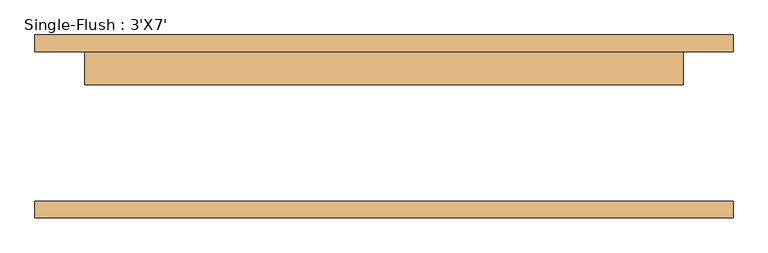
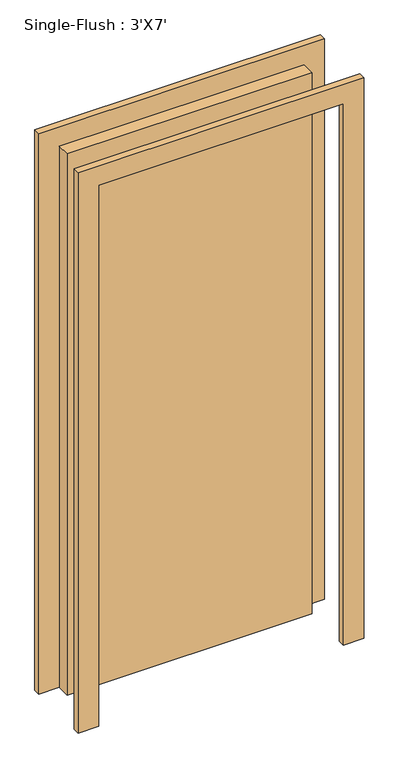
"""IFC4 building model written with IfcOpenShell, lengths in millimetres: door geometry, Single-Flush : 3'X7'."""

from ifc_helpers import new_model, si_unit, frame, origin, origin_with_axes, place, context, project, spatial, polyline, outline, extrude, source, transform, mapped, element, save


def single_flush_3_x7_0ca8825f(model_context):
    return source(origin(), model_context, "Body", "SweptSolid", [
        extrude(outline(polyline([(2209.8, -533.4), (0.0, -533.4), (0.0, -457.2), (2133.6, -457.2), (2133.6, 457.2), (0.0, 457.2), (0.0, 533.4), (2209.8, 533.4), (2209.8, -533.4)])), frame((0.0, 114.3, 0.0), z_axis=(0.0, 1.0, 0.0), x_axis=(0.0, 0.0, 1.0)), (0.0, 0.0, 1.0), 25.4),
        extrude(outline(polyline([(2209.8, 533.4), (2209.8, -533.4), (0.0, -533.4), (0.0, -457.2), (2133.6, -457.2), (2133.6, 457.2), (0.0, 457.2), (0.0, 533.4), (2209.8, 533.4)])), frame((0.0, -139.7, 0.0), z_axis=(0.0, 1.0, 0.0), x_axis=(0.0, 0.0, 1.0)), (0.0, 0.0, 1.0), 25.4),
        extrude(outline(polyline([(457.2, 63.5), (-457.2, 63.5), (-457.2, 114.3), (457.2, 114.3), (457.2, 63.5)])), origin_with_axes(), (0.0, 0.0, 1.0), 2133.6),
    ])


if __name__ == "__main__":
    model = new_model("IFC4")
    model_context = context("Model", 3, world=origin())
    ifc_project = project(units=[si_unit("LENGTHUNIT", "METRE", prefix="MILLI")], contexts=[model_context])
    site = spatial("IfcSite", under=ifc_project)
    building = spatial("IfcBuilding", under=site)
    placement = place(None, origin())
    single_flush_3_x7_shape = single_flush_3_x7_0ca8825f(model_context)
    element("IfcDoor", 1, ObjectType="Single-Flush : 3'X7'", at=placement, inside=building, context=model_context, shape_type="MappedRepresentation", body=[
        mapped(single_flush_3_x7_shape, transform((0.0, 0.0, 0.0), x_axis=(1.0, 0.0, 0.0), y_axis=(0.0, 1.0, 0.0), z_axis=(0.0, 0.0, 1.0))),
    ])
    save(model, "model.ifc")

# Revit data of these elements
# Type "Single-Flush : 3'X7'"
#   Type Mark = "8"
#   Construction Type Id = "MDOOR"
#   Assembly Code = "C1020"
#   Analytic Construction = "Metal"
#   Thickness = 0' - 2"
#   Heat Transfer Coefficient (U) = 0.651978 BTU/(h·ft²·°F)
#   Height = 7' - 0"
#   Trim Projection Ext = 0' - 1"
#   Trim Projection Int = 0' - 1"
#   Trim Width = 0' - 3"
#   Width = 3' - 0"
#   Define Thermal Properties by = 1
#   Door Material = Door - Panel
#   Frame Material = Door - Frame
#   Visual Light Transmittance = 0
#   Solar Heat Gain Coefficient = 0
#   Function = (empty or 0)
#   Wall Closure = (empty or 0)
# Element 1 (IfcDoor, "Single-Flush : 3'X7'")
#   Materials on its faces: "Door - Frame", "Door - Panel"
# Materials
#   "Door - Panel": class "Wood", colour RGB 210 159 95, transparency 0, Cost = 0
#   "Door - Frame": colour RGB 118 70 51, transparency 0, Cost = 0
